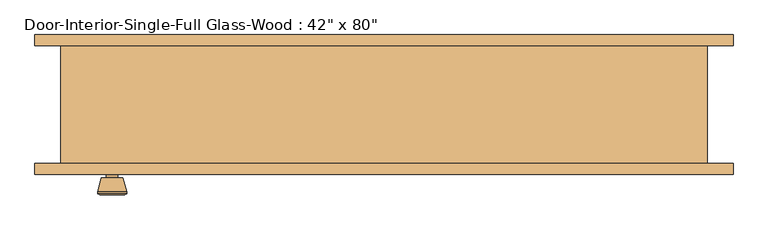
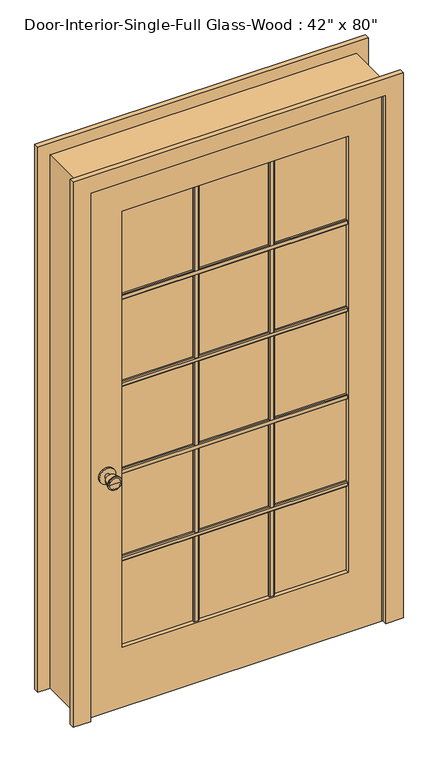
"""IFC4 building model written with IfcOpenShell, lengths in millimetres: door geometry."""

from ifc_helpers import new_model, si_unit, point, frame, frame_2d, origin, place, context, project, spatial, polyline, circle_curve, trimmed, segment, composite_curve, outline, extrude, faceted_brep, source, transform, mapped, element, save
from ifc_brep_helpers import plane_surface, cylinder_surface, revolved_surface, advanced_brep


def door_1d83da25(model_context):
    return source(origin(), model_context, "Body", "SolidModel", [
        extrude(outline(polyline([(-84.455, 1586.23), (-84.455, 1567.18), (-90.805, 1567.18), (-93.98, 1570.355), (-93.98, 1583.055), (-90.805, 1586.23), (-84.455, 1586.23)])), frame((-412.75, 0.0, 0.0), z_axis=(1.0, 0.0, 0.0), x_axis=(0.0, 1.0, 0.0)), (0.0, 0.0, 1.0), 825.5),
        extrude(outline(polyline([(-84.455, 1249.9975), (-84.455, 1230.9475), (-90.805, 1230.9475), (-93.98, 1234.1225), (-93.98, 1246.8225), (-90.805, 1249.9975), (-84.455, 1249.9975)])), frame((-412.75, 0.0, 0.0), z_axis=(1.0, 0.0, 0.0), x_axis=(0.0, 1.0, 0.0)), (0.0, 0.0, 1.0), 825.5),
        extrude(outline(polyline([(-84.455, 913.765), (-84.455, 894.715), (-90.805, 894.715), (-93.98, 897.89), (-93.98, 910.59), (-90.805, 913.765), (-84.455, 913.765)])), frame((-412.75, 0.0, 0.0), z_axis=(1.0, 0.0, 0.0), x_axis=(0.0, 1.0, 0.0)), (0.0, 0.0, 1.0), 825.5),
        extrude(outline(polyline([(-84.455, 577.5325), (-84.455, 558.4825), (-90.805, 558.4825), (-93.98, 561.6575), (-93.98, 574.3575), (-90.805, 577.5325), (-84.455, 577.5325)])), frame((-412.75, 0.0, 0.0), z_axis=(1.0, 0.0, 0.0), x_axis=(0.0, 1.0, 0.0)), (0.0, 0.0, 1.0), 825.5),
        extrude(outline(polyline([(128.0583333, -84.455), (147.1083333, -84.455), (147.1083333, -90.805), (143.9333333, -93.98), (131.2333333, -93.98), (128.0583333, -90.805), (128.0583333, -84.455)])), frame((0.0, 0.0, 231.775), z_axis=(0.0, 0.0, 1.0), x_axis=(1.0, 0.0, 0.0)), (0.0, 0.0, 1.0), 1681.1625),
        extrude(outline(polyline([(-147.1083333, -84.455), (-128.0583333, -84.455), (-128.0583333, -90.805), (-131.2333333, -93.98), (-143.9333333, -93.98), (-147.1083333, -90.805), (-147.1083333, -84.455)])), frame((0.0, 0.0, 231.775), z_axis=(0.0, 0.0, 1.0), x_axis=(1.0, 0.0, 0.0)), (0.0, 0.0, 1.0), 1681.1625),
        extrude(outline(polyline([(-77.47, 1586.23), (-71.12, 1586.23), (-67.945, 1583.055), (-67.945, 1570.355), (-71.12, 1567.18), (-77.47, 1567.18), (-77.47, 1586.23)])), frame((-412.75, 0.0, 0.0), z_axis=(1.0, 0.0, 0.0), x_axis=(0.0, 1.0, 0.0)), (0.0, 0.0, 1.0), 825.5),
        extrude(outline(polyline([(-77.47, 1249.9975), (-71.12, 1249.9975), (-67.945, 1246.8225), (-67.945, 1234.1225), (-71.12, 1230.9475), (-77.47, 1230.9475), (-77.47, 1249.9975)])), frame((-412.75, 0.0, 0.0), z_axis=(1.0, 0.0, 0.0), x_axis=(0.0, 1.0, 0.0)), (0.0, 0.0, 1.0), 825.5),
        extrude(outline(polyline([(-77.47, 913.765), (-71.12, 913.765), (-67.945, 910.59), (-67.945, 897.89), (-71.12, 894.715), (-77.47, 894.715), (-77.47, 913.765)])), frame((-412.75, 0.0, 0.0), z_axis=(1.0, 0.0, 0.0), x_axis=(0.0, 1.0, 0.0)), (0.0, 0.0, 1.0), 825.5),
        extrude(outline(polyline([(-77.47, 577.5325), (-71.12, 577.5325), (-67.945, 574.3575), (-67.945, 561.6575), (-71.12, 558.4825), (-77.47, 558.4825), (-77.47, 577.5325)])), frame((-412.75, 0.0, 0.0), z_axis=(1.0, 0.0, 0.0), x_axis=(0.0, 1.0, 0.0)), (0.0, 0.0, 1.0), 825.5),
        extrude(outline(polyline([(128.0583333, -77.47), (128.0583333, -71.12), (131.2333333, -67.945), (143.9333333, -67.945), (147.1083333, -71.12), (147.1083333, -77.47), (128.0583333, -77.47)])), frame((0.0, 0.0, 231.775), z_axis=(0.0, 0.0, 1.0), x_axis=(1.0, 0.0, 0.0)), (0.0, 0.0, 1.0), 1681.1625),
        extrude(outline(polyline([(-147.1083333, -77.47), (-147.1083333, -71.12), (-143.9333333, -67.945), (-131.2333333, -67.945), (-128.0583333, -71.12), (-128.0583333, -77.47), (-147.1083333, -77.47)])), frame((0.0, 0.0, 231.775), z_axis=(0.0, 0.0, 1.0), x_axis=(1.0, 0.0, 0.0)), (0.0, 0.0, 1.0), 1681.1625),
        advanced_brep(
        [(-469.9, -57.5, 914.4), (-479.9, -57.5, 914.4), (-459.9, -57.5, 914.4), (-449.4241324, -8.5, 914.4), (-490.3758676, -8.5, 914.4), (-469.9, -8.5, 914.4), (-444.9, -10.3278681, 914.4), (-494.9, -10.3278681, 914.4), (-444.9, -13.7915463, 914.4), (-494.9, -13.7915463, 914.4), (-451.263764, -38.5, 914.4), (-488.536236, -38.5, 914.4), (-459.9, -38.5, 914.4), (-479.9, -38.5, 914.4)],
        [
            (0, 1),
            (1, 2, circle_curve(frame((-469.9, -57.5, 914.4), z_axis=(0.0, -1.0, 0.0), x_axis=(-1.0, 0.0, 0.0)), 10.0)),
            (2, 0),
            (2, 1, circle_curve(frame((-469.9, -57.5, 914.4), z_axis=(0.0, -1.0, 0.0), x_axis=(-1.0, 0.0, 0.0)), 10.0)),
            (3, 4, circle_curve(frame((-469.9, -8.5, 914.4), z_axis=(0.0, 1.0, 0.0), x_axis=(-1.0, 0.0, 0.0)), 20.4758676)),
            (4, 5),
            (5, 3),
            (4, 3, circle_curve(frame((-469.9, -8.5, 914.4), z_axis=(0.0, 1.0, 0.0), x_axis=(-1.0, 0.0, 0.0)), 20.4758676)),
            (6, 7, circle_curve(frame((-469.9, -10.3278681, 914.4), z_axis=(0.0, 1.0, 0.0), x_axis=(-1.0, 0.0, 0.0)), 25.0)),
            (7, 4),
            (3, 6),
            (7, 6, circle_curve(frame((-469.9, -10.3278681, 914.4), z_axis=(0.0, 1.0, 0.0), x_axis=(-1.0, 0.0, 0.0)), 25.0)),
            (8, 9, circle_curve(frame((-469.9, -13.7915463, 914.4), z_axis=(0.0, 1.0, 0.0), x_axis=(-1.0, 0.0, 0.0)), 25.0)),
            (9, 7),
            (6, 8),
            (9, 8, circle_curve(frame((-469.9, -13.7915463, 914.4), z_axis=(0.0, 1.0, 0.0), x_axis=(-1.0, 0.0, 0.0)), 25.0)),
            (10, 11, circle_curve(frame((-469.9, -38.5, 914.4), z_axis=(0.0, 1.0, 0.0), x_axis=(-1.0, 0.0, 0.0)), 18.636236)),
            (11, 9),
            (8, 10),
            (11, 10, circle_curve(frame((-469.9, -38.5, 914.4), z_axis=(0.0, 1.0, 0.0), x_axis=(-1.0, 0.0, 0.0)), 18.636236)),
            (12, 13, circle_curve(frame((-469.9, -38.5, 914.4), z_axis=(0.0, 1.0, 0.0), x_axis=(-1.0, 0.0, 0.0)), 10.0)),
            (13, 11),
            (10, 12),
            (13, 12, circle_curve(frame((-469.9, -38.5, 914.4), z_axis=(0.0, 1.0, 0.0), x_axis=(-1.0, 0.0, 0.0)), 10.0)),
            (1, 13),
            (12, 2),
        ],
        [
            plane_surface(frame((-469.9, -57.5, 914.4), z_axis=(0.0, -1.0, 0.0), x_axis=(-1.0, 0.0, 0.0))),
            plane_surface(frame((-469.9, -8.5, 914.4), z_axis=(0.0, 1.0, 0.0), x_axis=(-1.0, 0.0, 0.0))),
            revolved_surface(polyline([(-490.3758676, -8.5, 914.4), (-494.9, -10.3278681, 914.4)]), (-469.9, -57.5, 914.4), (0.0, -1.0, 0.0)),
            cylinder_surface(frame((-469.9, -57.5, 914.4), z_axis=(0.0, -1.0, 0.0), x_axis=(-1.0, 0.0, 0.0)), 25.0),
            revolved_surface(polyline([(-494.9, -13.7915463, 914.4), (-488.536236, -38.5, 914.4)]), (-469.9, -57.5, 914.4), (0.0, -1.0, 0.0)),
            plane_surface(frame((-469.9, -38.5, 914.4), z_axis=(0.0, -1.0, 0.0), x_axis=(-1.0, 0.0, 0.0))),
            cylinder_surface(frame((-469.9, -57.5, 914.4), z_axis=(0.0, -1.0, 0.0), x_axis=(-1.0, 0.0, 0.0)), 10.0),
        ],
        [
            (0, [[1, 2, 3]]),
            (0, [[-3, 4, -1]]),
            (1, [[5, 6, 7]]),
            (1, [[8, -7, -6]]),
            (2, [[9, 10, -5, 11]]),
            (2, [[12, -11, -8, -10]]),
            (3, [[13, 14, -9, 15]]),
            (3, [[16, -15, -12, -14]]),
            (4, [[17, 18, -13, 19]]),
            (4, [[20, -19, -16, -18]]),
            (5, [[21, 22, -17, 23]]),
            (5, [[24, -23, -20, -22]]),
            (6, [[-2, 25, -21, 26]]),
            (6, [[-4, -26, -24, -25]]),
        ],
    ),
        extrude(outline(composite_curve([segment(trimmed(circle_curve(frame_2d((914.4, -469.9)), 30.0), [point((914.4, -499.9))], [point((914.4, -439.9))], False, "CARTESIAN"), True, "CONTINUOUS"), segment(trimmed(circle_curve(frame_2d((914.4, -469.9)), 30.0), [point((914.4, -439.9))], [point((914.4, -499.9))], False, "CARTESIAN"), True, "CONTINUOUS")], self_intersect=False)), frame((0.0, -63.5, 0.0), z_axis=(0.0, 1.0, 0.0), x_axis=(0.0, 0.0, 1.0)), (0.0, 0.0, 1.0), 6.0),
        advanced_brep(
        [(-469.9, -104.425, 914.4), (-459.9, -104.425, 914.4), (-479.9, -104.425, 914.4), (-449.4241324, -153.425, 914.4), (-469.9, -153.425, 914.4), (-490.3758676, -153.425, 914.4), (-444.9, -151.5971319, 914.4), (-494.9, -151.5971319, 914.4), (-444.9, -148.1334537, 914.4), (-494.9, -148.1334537, 914.4), (-451.263764, -123.425, 914.4), (-488.536236, -123.425, 914.4), (-459.9, -123.425, 914.4), (-479.9, -123.425, 914.4)],
        [
            (0, 1),
            (1, 2, circle_curve(frame((-469.9, -104.425, 914.4), z_axis=(0.0, 1.0, 0.0), x_axis=(-1.0, 0.0, 0.0)), 10.0)),
            (2, 0),
            (2, 1, circle_curve(frame((-469.9, -104.425, 914.4), z_axis=(0.0, 1.0, 0.0), x_axis=(-1.0, 0.0, 0.0)), 10.0)),
            (3, 4),
            (4, 5),
            (5, 3, circle_curve(frame((-469.9, -153.425, 914.4), z_axis=(0.0, -1.0, 0.0), x_axis=(-1.0, 0.0, 0.0)), 20.4758676)),
            (3, 5, circle_curve(frame((-469.9, -153.425, 914.4), z_axis=(0.0, -1.0, 0.0), x_axis=(-1.0, 0.0, 0.0)), 20.4758676)),
            (6, 3),
            (5, 7),
            (7, 6, circle_curve(frame((-469.9, -151.5971319, 914.4), z_axis=(0.0, -1.0, 0.0), x_axis=(-1.0, 0.0, 0.0)), 25.0)),
            (6, 7, circle_curve(frame((-469.9, -151.5971319, 914.4), z_axis=(0.0, -1.0, 0.0), x_axis=(-1.0, 0.0, 0.0)), 25.0)),
            (8, 6),
            (7, 9),
            (9, 8, circle_curve(frame((-469.9, -148.1334537, 914.4), z_axis=(0.0, -1.0, 0.0), x_axis=(-1.0, 0.0, 0.0)), 25.0)),
            (8, 9, circle_curve(frame((-469.9, -148.1334537, 914.4), z_axis=(0.0, -1.0, 0.0), x_axis=(-1.0, 0.0, 0.0)), 25.0)),
            (10, 8),
            (9, 11),
            (11, 10, circle_curve(frame((-469.9, -123.425, 914.4), z_axis=(0.0, -1.0, 0.0), x_axis=(-1.0, 0.0, 0.0)), 18.636236)),
            (10, 11, circle_curve(frame((-469.9, -123.425, 914.4), z_axis=(0.0, -1.0, 0.0), x_axis=(-1.0, 0.0, 0.0)), 18.636236)),
            (12, 10),
            (11, 13),
            (13, 12, circle_curve(frame((-469.9, -123.425, 914.4), z_axis=(0.0, -1.0, 0.0), x_axis=(-1.0, 0.0, 0.0)), 10.0)),
            (12, 13, circle_curve(frame((-469.9, -123.425, 914.4), z_axis=(0.0, -1.0, 0.0), x_axis=(-1.0, 0.0, 0.0)), 10.0)),
            (1, 12),
            (13, 2),
        ],
        [
            plane_surface(frame((-469.9, -104.425, 914.4), z_axis=(0.0, 1.0, 0.0), x_axis=(-1.0, 0.0, 0.0))),
            plane_surface(frame((-469.9, -153.425, 914.4), z_axis=(0.0, -1.0, 0.0), x_axis=(-1.0, 0.0, 0.0))),
            revolved_surface(polyline([(-490.3758676, -153.425, 914.4), (-494.9, -151.5971319, 914.4)]), (-469.9, -104.425, 914.4), (0.0, 1.0, 0.0)),
            cylinder_surface(frame((-469.9, -104.425, 914.4), z_axis=(0.0, 1.0, 0.0), x_axis=(-1.0, 0.0, 0.0)), 25.0),
            revolved_surface(polyline([(-494.9, -148.1334537, 914.4), (-488.536236, -123.425, 914.4)]), (-469.9, -104.425, 914.4), (0.0, 1.0, 0.0)),
            plane_surface(frame((-469.9, -123.425, 914.4), z_axis=(0.0, 1.0, 0.0), x_axis=(-1.0, 0.0, 0.0))),
            cylinder_surface(frame((-469.9, -104.425, 914.4), z_axis=(0.0, 1.0, 0.0), x_axis=(-1.0, 0.0, 0.0)), 10.0),
        ],
        [
            (0, [[1, 2, 3]]),
            (0, [[-3, 4, -1]]),
            (1, [[5, 6, 7]]),
            (1, [[-6, -5, 8]]),
            (2, [[9, -7, 10, 11]]),
            (2, [[-10, -8, -9, 12]]),
            (3, [[13, -11, 14, 15]]),
            (3, [[-14, -12, -13, 16]]),
            (4, [[17, -15, 18, 19]]),
            (4, [[-18, -16, -17, 20]]),
            (5, [[21, -19, 22, 23]]),
            (5, [[-22, -20, -21, 24]]),
            (6, [[25, -23, 26, -2]]),
            (6, [[-26, -24, -25, -4]]),
        ],
    ),
        extrude(outline(composite_curve([segment(trimmed(circle_curve(frame_2d((914.4, -469.9)), 30.0), [point((914.4, -499.9))], [point((914.4, -439.9))], False, "CARTESIAN"), True, "CONTINUOUS"), segment(trimmed(circle_curve(frame_2d((914.4, -469.9)), 30.0), [point((914.4, -439.9))], [point((914.4, -499.9))], False, "CARTESIAN"), True, "CONTINUOUS")], self_intersect=False)), frame((0.0, -104.425, 0.0), z_axis=(0.0, 1.0, 0.0), x_axis=(0.0, 0.0, 1.0)), (0.0, 0.0, 1.0), 6.0),
        extrude(outline(polyline([(2032.0, -533.4), (0.0, -533.4), (0.0, 533.4), (2032.0, 533.4), (2032.0, -533.4)]), holes=[polyline([(1912.9375, -412.75), (1912.9375, 412.75), (231.775, 412.75), (231.775, -412.75), (1912.9375, -412.75)])]), frame((0.0, -98.425, 0.0), z_axis=(0.0, 1.0, 0.0), x_axis=(0.0, 0.0, 1.0)), (0.0, 0.0, 1.0), 34.925),
        faceted_brep([(558.8, -98.425, 0.0), (533.4, -98.425, 0.0), (533.4, -63.5, 0.0), (520.7, -63.5, 0.0), (520.7, -28.575, 0.0), (533.4, -28.575, 0.0), (533.4, 104.775, 0.0), (558.8, 104.775, 0.0), (558.8, 104.775, 2057.4), (558.8, -98.425, 2057.4), (533.4, 104.775, 2032.0), (-533.4, 104.775, 2032.0), (-533.4, 104.775, 0.0), (-558.8, 104.775, 0.0), (-558.8, 104.775, 2057.4), (533.4, -28.575, 2032.0), (520.7, -28.575, 2019.3), (-520.7, -28.575, 2019.3), (-520.7, -28.575, 0.0), (-533.4, -28.575, 0.0), (-533.4, -28.575, 2032.0), (520.7, -63.5, 2019.3), (533.4, -63.5, 2032.0), (-533.4, -63.5, 2032.0), (-533.4, -63.5, 0.0), (-520.7, -63.5, 0.0), (-520.7, -63.5, 2019.3), (533.4, -98.425, 2032.0), (-558.8, -98.425, 2057.4), (-558.8, -98.425, 0.0), (-533.4, -98.425, 0.0), (-533.4, -98.425, 2032.0)], [[[0, 1, 2, 3, 4, 5, 6, 7]], [[7, 8, 9, 0]], [[6, 10, 11, 12, 13, 14, 8, 7]], [[5, 15, 10, 6]], [[4, 16, 17, 18, 19, 20, 15, 5]], [[3, 21, 16, 4]], [[2, 22, 23, 24, 25, 26, 21, 3]], [[1, 27, 22, 2]], [[0, 9, 28, 29, 30, 31, 27, 1]], [[8, 14, 28, 9]], [[15, 20, 11, 10]], [[21, 26, 17, 16]], [[27, 31, 23, 22]], [[29, 13, 12, 19, 18, 25, 24, 30]], [[14, 13, 29, 28]], [[20, 19, 12, 11]], [[26, 25, 18, 17]], [[31, 30, 24, 23]]]),
        extrude(outline(polyline([(412.75, -77.47), (412.75, -84.455), (-412.75, -84.455), (-412.75, -77.47), (412.75, -77.47)])), frame((0.0, 0.0, 231.775), z_axis=(0.0, 0.0, 1.0), x_axis=(1.0, 0.0, 0.0)), (0.0, 0.0, 1.0), 1681.1625),
        extrude(outline(polyline([(0.0, 603.25), (2101.85, 603.25), (2101.85, -603.25), (0.0, -603.25), (0.0, -539.75), (2038.35, -539.75), (2038.35, 539.75), (0.0, 539.75), (0.0, 603.25)])), frame((0.0, 104.775, 0.0), z_axis=(0.0, 1.0, 0.0), x_axis=(0.0, 0.0, 1.0)), (0.0, 0.0, 1.0), 19.05),
        extrude(outline(polyline([(0.0, 603.25), (2101.85, 603.25), (2101.85, -603.25), (0.0, -603.25), (0.0, -539.75), (2038.35, -539.75), (2038.35, 539.75), (0.0, 539.75), (0.0, 603.25)])), frame((0.0, -117.475, 0.0), z_axis=(0.0, 1.0, 0.0), x_axis=(0.0, 0.0, 1.0)), (0.0, 0.0, 1.0), 19.05),
    ])


if __name__ == "__main__":
    model = new_model("IFC4")
    model_context = context("Model", 3, world=origin())
    ifc_project = project(units=[si_unit("LENGTHUNIT", "METRE", prefix="MILLI")], contexts=[model_context])
    site = spatial("IfcSite", under=ifc_project)
    building = spatial("IfcBuilding", under=site)
    placement = place(None, origin())
    door_shape = door_1d83da25(model_context)
    element("IfcDoor", 1, ObjectType="Door-Interior-Single-Full Glass-Wood : 42\" x 80\"", at=placement, inside=building, context=model_context, shape_type="MappedRepresentation", body=[
        mapped(door_shape, transform((0.0, 0.0, 0.0), x_axis=(1.0, 0.0, 0.0), y_axis=(0.0, 1.0, 0.0), z_axis=(0.0, 0.0, 1.0))),
    ])
    save(model, "model.ifc")

# Revit data of these elements
# Type "Door-Interior-Single-Full Glass-Wood : 42\" x 80\""
#   Type Mark = "10"
#   Assembly Code = "C1020300"
#   Analytic Construction = "Wood frame with single clear glass"
#   Top Rail = 0' - 4 11/16"
#   Thickness = 0' - 1 3/8"
#   Thermal Resistance (R) = 1.0102 (h·ft²·°F)/BTU
#   Swing Angle [instance default] = 90.00°
#   Stiles = 0' - 4 3/4"
#   Rough Width = 3' - 8"
#   Rough Height = 6' - 9"
#   Height = 6' - 8"
#   Width = 3' - 6"
#   Heat Transfer Coefficient (U) = 0.9900 BTU/(h·ft²·°F)
#   Bottom Rail = 0' - 9 1/8"
#   Show Grill [instance default] = yes
#   Trim Material = Cherry
#   Panel Material = Cherry
#   Frame Material = Cherry
#   Door Handle Material = Aluminum
#   Visual Light Transmittance = 0
#   Solar Heat Gain Coefficient = 0
#   Wall Closure = (empty or 0)
#   Function = (empty or 0)
# Element 1 (IfcDoor, "Door-Interior-Single-Full Glass-Wood : 42\" x 80\"")
#   Materials on its faces: "Cherry", "Aluminum", "Glass"
# Materials
#   "Cherry": class "Wood", colour RGB 226 177 128, transparency 0, Description = "Prunus Serotina", Cost = 0
#   "Aluminum": class "Metal", colour RGB 247 247 247, transparency 0, Description = "Aluminum 6061", Cost = 0
#   "Glass": class "Glass", colour RGB 0 128 192, transparency 0.75, Description = "Soda Lime Glass", Cost = 0
